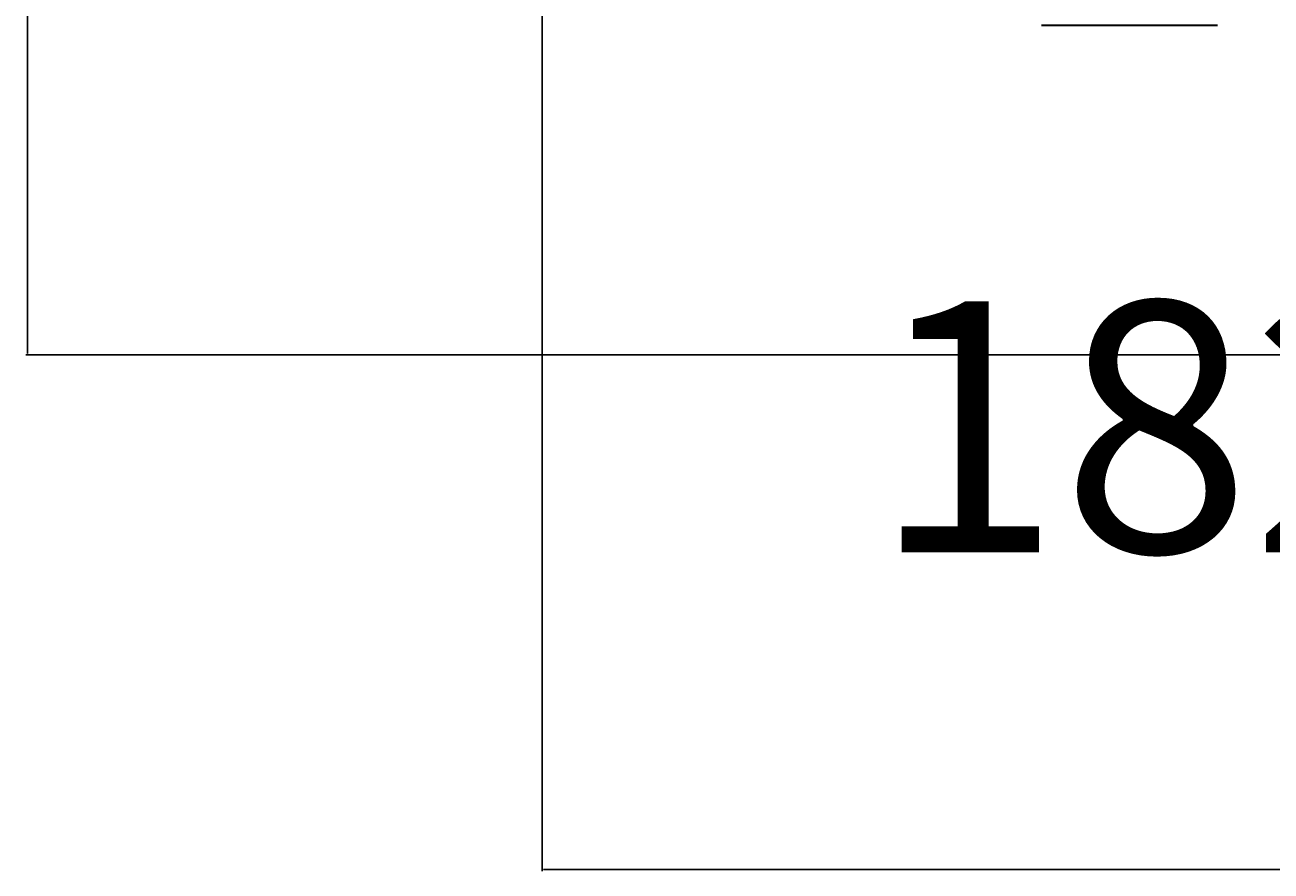
# Model space of a CAD drawing. Units: millimetres. Extents: x 27017497 to 27018854, y 7058029 to 7059154.
# Tile 1 of 91: x 27017497 to 27017651, y 7058029 to 7058133. Entities that reach past the tile are written whole.
import ezdxf

# ---------------------------------------------------------------- set-up
doc = ezdxf.new("R2010")
doc.units = ezdxf.units.MM
for name, color, linetype, lineweight in [('A-ANNO-DIMS', 2, 'Continuous', 18), ('A-AREA-IDEN', 7, 'Continuous', 18), ('A-WALL', 7, 'Continuous', 35)]:
    doc.layers.add(name, color=color, linetype=linetype, lineweight=lineweight)
doc.styles.get("Standard").update_dxf_attribs({"font": 'arial.ttf'})
doc.dimstyles.get("Standard").update_dxf_attribs({"dimtxt": 0.18, "dimasz": 0.18, "dimexe": 0.18, "dimexo": 0.0625, "dimgap": 0.09, "dimtad": 0, "dimtih": 1, "dimtoh": 1, "dimdec": 4, "dimzin": 0, "dimdsep": 46, "dimtxsty": 'Standard', "dimcen": 0.09, "dimadec": 0, "dimazin": 0, "dimtfac": 1, "dimtdec": 4, "dimtofl": 0, "dimtmove": 0, "dimatfit": 3, "dimfxl": 1, "dimtolj": 1, "dimtzin": 0, "dimarcsym": 0})

# ---------------------------------------------------------------- blocks, each defined once
blk = doc.blocks.new('*D47')
at = {"layer": 'A-ANNO-DIMS', "color": 0, "lineweight": -2, "transparency": 16777216}
for p, q in [((27017561.17, 7058294.35), (27017561.17, 7058028.6)), ((27018790.61, 7058294.35), (27018790.61, 7058028.6)), ((27017561.35, 7058028.78), (27018175.43, 7058028.78)), ((27018790.43, 7058028.78), (27018176.34, 7058028.78))]:
    blk.add_line(p, q, dxfattribs=at)
at = {"layer": 'A-ANNO-DIMS', "color": 0, "transparency": 16777216}
for points in [[(27017561.35, 7058028.81), (27017561.35, 7058028.75), (27017561.17, 7058028.78)], [(27018790.43, 7058028.81), (27018790.43, 7058028.75), (27018790.61, 7058028.78)]]:
    blk.add_solid(points, dxfattribs=at)
at = {"layer": 'Defpoints', "color": 0, "transparency": 16777216}
for p in [(27017561.17, 7058294.41), (27018790.61, 7058294.41), (27018790.61, 7058028.78)]:
    blk.add_point(p, dxfattribs=at)
at = {"layer": 'A-ANNO-DIMS', "color": 0, "transparency": 16777216, "insert": (27018175.89, 7058028.78), "char_height": 0.18, "attachment_point": 5}
blk.add_mtext('\\A1;1229.4', dxfattribs=at)
blk = doc.blocks.new('*D48')
at = {"layer": 'A-ANNO-DIMS', "color": 0, "lineweight": -2, "transparency": 16777216}
for p, q in [((27018463.5, 7058622.91), (27017497.54, 7058622.91)), ((27017497.72, 7058622.73), (27017497.72, 7058357.75)), ((27017497.72, 7058092.41), (27017497.72, 7058357.39)), ((27018555.13, 7058092.23), (27017497.54, 7058092.23))]:
    blk.add_line(p, q, dxfattribs=at)
at = {"layer": 'A-ANNO-DIMS', "color": 0, "transparency": 16777216}
for points in [[(27017497.69, 7058622.73), (27017497.75, 7058622.73), (27017497.72, 7058622.91)], [(27017497.69, 7058092.41), (27017497.75, 7058092.41), (27017497.72, 7058092.23)]]:
    blk.add_solid(points, dxfattribs=at)
at = {"layer": 'Defpoints', "color": 0, "transparency": 16777216}
for p in [(27018463.56, 7058622.91), (27017497.72, 7058092.23), (27018555.19, 7058092.23)]:
    blk.add_point(p, dxfattribs=at)
at = {"layer": 'A-ANNO-DIMS', "color": 0, "transparency": 16777216, "insert": (27017497.72, 7058357.57), "char_height": 0.18, "attachment_point": 5}
blk.add_mtext('\\A1;530.7', dxfattribs=at)

msp = doc.modelspace()

# ---------------------------------------------------------------- linework, layer by layer
at = {"layer": 'A-WALL'}
msp.add_line((27017622.724, 7058132.888), (27017644.461, 7058132.888), dxfattribs=at)

# ---------------------------------------------------------------- texts
at = {"layer": 'A-AREA-IDEN'}
msp.add_text('1824SFT', height=30.9043, dxfattribs=at).set_placement((27017601.779, 7058067.907))

# ---------------------------------------------------------------- dimensions: what is measured, and where the dimension line sits
at = {"layer": 'A-ANNO-DIMS'}
dim = msp.add_linear_dim(base=(27017497.716, 7058092.23), p1=(27018463.561, 7058622.912), p2=(27018555.192, 7058092.23), angle=90, dimstyle='Standard', override={"dimdec": 1, "dimlfac": 1, "dimrnd": 0, "dimzin": 0, "dimdsep": 46, "dimlunit": 2}, dxfattribs=at)
dim.commit()
dim.dimension.update_dxf_attribs({"geometry": '*D48', "text_midpoint": (27017497.716, 7058357.571)})
dim = msp.add_linear_dim(base=(27018790.606, 7058028.78), p1=(27017561.166, 7058294.412), p2=(27018790.606, 7058294.412), dimstyle='Standard', override={"dimdec": 1, "dimlfac": 1, "dimrnd": 0, "dimzin": 0, "dimdsep": 46, "dimlunit": 2}, dxfattribs=at)
dim.commit()
dim.dimension.update_dxf_attribs({"geometry": '*D47', "text_midpoint": (27018175.886, 7058028.78)})

doc.saveas('drawing.dxf')
